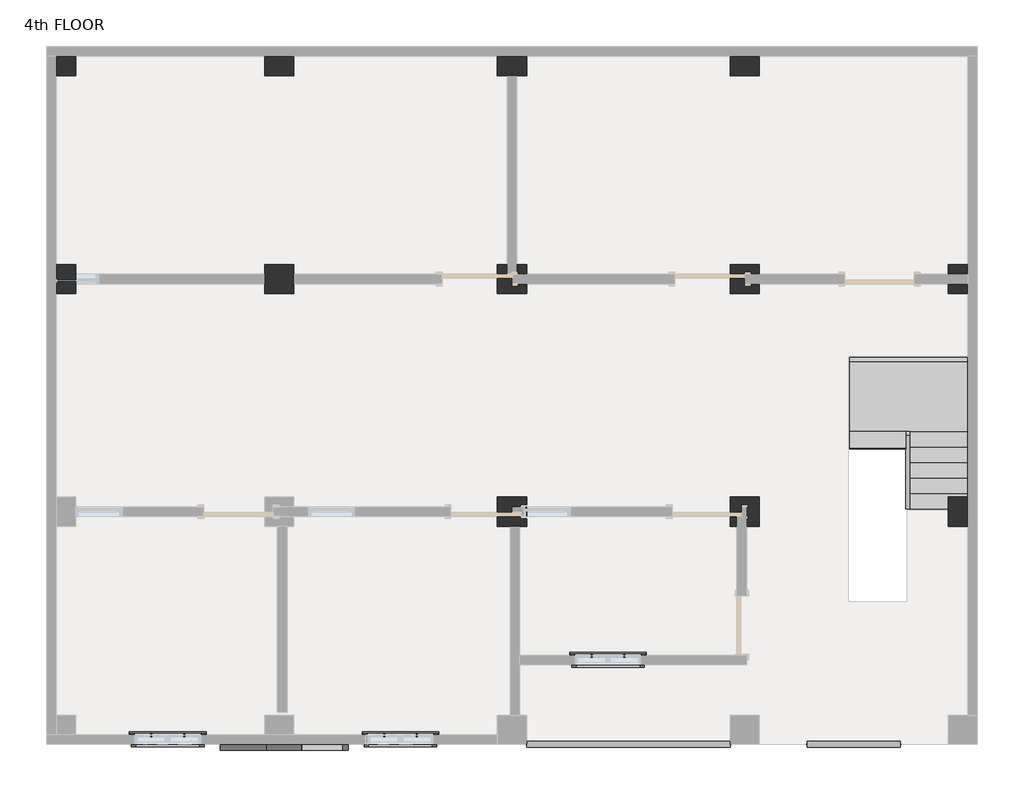
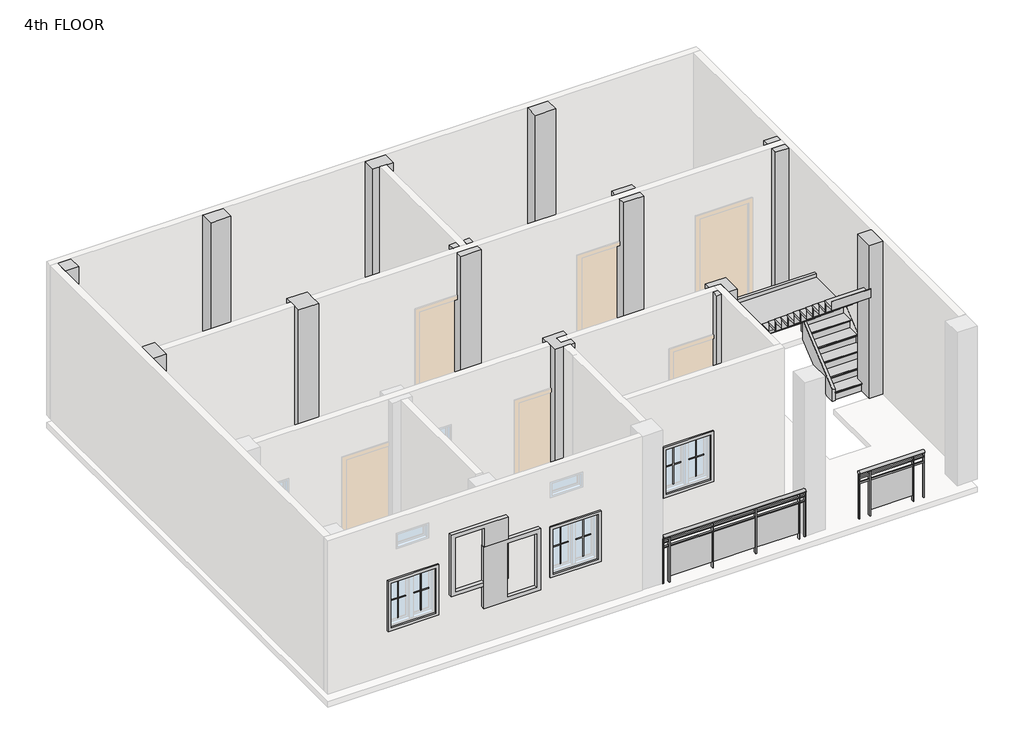
# One storey, part 2 of 2: 12 columns, 12 proxies, 4 members, 2 railings, 1 damper, 1 stair flight.
"""IFC4 building model written with IfcOpenShell, lengths in millimetres."""

from ifc_helpers import new_model, si_unit, point, frame, origin, place, context, project, spatial, polyline, ellipse_curve, trimmed, outline, extrude, faceted_brep, transform, mapped, element, save
from ifc_brep_helpers import plane_surface, extruded_surface, advanced_brep
from components import muntin_pattern_2x2_muntin_pattern_2x2_b3fe6957, muntin_pattern_2x2_muntin_pattern_2x2_3e0ecaf2, trim_window_exterior_flat_with_sill_41619996, trim_window_interior_flat_picture_frame_51c85655, duct_accessories_9_duct_accessories_1_ba76d1db, stair_flight_b92ce0aa

model = new_model("IFC4")

# Units and contexts
model_context = context("Model", 3, world=origin())
ifc_project = project(units=[si_unit("LENGTHUNIT", "METRE", prefix="MILLI")], contexts=[model_context])

# Site, building, storey
site = spatial("IfcSite", under=ifc_project)
building = spatial("IfcBuilding", under=site)
storey = spatial("IfcBuildingStorey", under=building, Name="4th FLOOR", Elevation=12039.6)

# Proxies
placement = place(None, origin())
muntin_pattern_2x2_muntin_pattern_2x2_shape = muntin_pattern_2x2_muntin_pattern_2x2_b3fe6957(model_context)
element("IfcBuildingElementProxy", 1, Name="Muntin Pattern_2x2 : Muntin Pattern_2x2", ObjectType="Muntin Pattern_2x2 : Muntin Pattern_2x2", at=placement, inside=storey, context=model_context, shape_type="MappedRepresentation", body=[
    mapped(muntin_pattern_2x2_muntin_pattern_2x2_shape, transform((-14441.409625, -253.8184478, 13023.85), x_axis=(1.0, 0.0, 0.0), y_axis=(0.0, 1.0, 0.0), z_axis=(0.0, 0.0, 1.0))),
])
element("IfcBuildingElementProxy", 2, Name="Muntin Pattern_2x2 : Muntin Pattern_2x2", ObjectType="Muntin Pattern_2x2 : Muntin Pattern_2x2", at=placement, inside=storey, context=model_context, shape_type="MappedRepresentation", body=[
    mapped(muntin_pattern_2x2_muntin_pattern_2x2_shape, transform((-11393.409625, -253.8184478, 13023.85), x_axis=(1.0, 0.0, 0.0), y_axis=(0.0, 1.0, 0.0), z_axis=(0.0, 0.0, 1.0))),
])
element("IfcBuildingElementProxy", 3, Name="Muntin Pattern_2x2 : Muntin Pattern_2x2", ObjectType="Muntin Pattern_2x2 : Muntin Pattern_2x2", at=placement, inside=storey, context=model_context, shape_type="MappedRepresentation", body=[
    mapped(muntin_pattern_2x2_muntin_pattern_2x2_shape, transform((-8675.609625, 787.5815522, 13023.85), x_axis=(1.0, 0.0, 0.0), y_axis=(0.0, 1.0, 0.0), z_axis=(0.0, 0.0, 1.0))),
])
muntin_pattern_2x2_muntin_pattern_2x2_2_shape = muntin_pattern_2x2_muntin_pattern_2x2_3e0ecaf2(model_context)
element("IfcBuildingElementProxy", 4, Name="Muntin Pattern_2x2 : Muntin Pattern_2x2", ObjectType="Muntin Pattern_2x2 : Muntin Pattern_2x2", at=placement, inside=storey, context=model_context, shape_type="MappedRepresentation", body=[
    mapped(muntin_pattern_2x2_muntin_pattern_2x2_2_shape, transform((-14012.784625, -253.8184478, 13023.85), x_axis=(-1.0, 0.0, 0.0), y_axis=(0.0, -1.0, 0.0), z_axis=(0.0, 0.0, 1.0))),
])
element("IfcBuildingElementProxy", 5, Name="Muntin Pattern_2x2 : Muntin Pattern_2x2", ObjectType="Muntin Pattern_2x2 : Muntin Pattern_2x2", at=placement, inside=storey, context=model_context, shape_type="MappedRepresentation", body=[
    mapped(muntin_pattern_2x2_muntin_pattern_2x2_2_shape, transform((-10964.784625, -253.8184478, 13023.85), x_axis=(-1.0, 0.0, 0.0), y_axis=(0.0, -1.0, 0.0), z_axis=(0.0, 0.0, 1.0))),
])
element("IfcBuildingElementProxy", 6, Name="Muntin Pattern_2x2 : Muntin Pattern_2x2", ObjectType="Muntin Pattern_2x2 : Muntin Pattern_2x2", at=placement, inside=storey, context=model_context, shape_type="MappedRepresentation", body=[
    mapped(muntin_pattern_2x2_muntin_pattern_2x2_2_shape, transform((-8246.984625, 787.5815522, 13023.85), x_axis=(-1.0, 0.0, 0.0), y_axis=(0.0, -1.0, 0.0), z_axis=(0.0, 0.0, 1.0))),
])
trim_window_exterior_flat_with_sill_shape = trim_window_exterior_flat_with_sill_41619996(model_context)
element("IfcBuildingElementProxy", 7, Name="Trim-Window-Exterior-Flat : with Sill", ObjectType="Trim-Window-Exterior-Flat : with Sill", at=placement, inside=storey, context=model_context, shape_type="MappedRepresentation", body=[
    mapped(trim_window_exterior_flat_with_sill_shape, transform((-14227.097125, -244.2934478, 13868.4), x_axis=(-1.0, 0.0, 0.0), y_axis=(0.0, 0.0, 1.0), z_axis=(0.0, 1.0, 0.0))),
])
element("IfcBuildingElementProxy", 8, Name="Trim-Window-Exterior-Flat : with Sill", ObjectType="Trim-Window-Exterior-Flat : with Sill", at=placement, inside=storey, context=model_context, shape_type="MappedRepresentation", body=[
    mapped(trim_window_exterior_flat_with_sill_shape, transform((-11179.097125, -244.2934478, 13868.4), x_axis=(-1.0, 0.0, 0.0), y_axis=(0.0, 0.0, 1.0), z_axis=(0.0, 1.0, 0.0))),
])
element("IfcBuildingElementProxy", 9, Name="Trim-Window-Exterior-Flat : with Sill", ObjectType="Trim-Window-Exterior-Flat : with Sill", at=placement, inside=storey, context=model_context, shape_type="MappedRepresentation", body=[
    mapped(trim_window_exterior_flat_with_sill_shape, transform((-8461.297125, 797.1065522, 13868.4), x_axis=(-1.0, 0.0, 0.0), y_axis=(0.0, 0.0, 1.0), z_axis=(0.0, 1.0, 0.0))),
])
trim_window_interior_flat_picture_frame_shape = trim_window_interior_flat_picture_frame_51c85655(model_context)
element("IfcBuildingElementProxy", 10, Name="Trim-Window-Interior-Flat : Picture Frame", ObjectType="Trim-Window-Interior-Flat : Picture Frame", at=placement, inside=storey, context=model_context, shape_type="MappedRepresentation", body=[
    mapped(trim_window_interior_flat_picture_frame_shape, transform((-14227.097125, -371.2934478, 13868.4), x_axis=(1.0, 0.0, 0.0), y_axis=(0.0, 0.0, 1.0), z_axis=(0.0, -1.0, 0.0))),
])
element("IfcBuildingElementProxy", 11, Name="Trim-Window-Interior-Flat : Picture Frame", ObjectType="Trim-Window-Interior-Flat : Picture Frame", at=placement, inside=storey, context=model_context, shape_type="MappedRepresentation", body=[
    mapped(trim_window_interior_flat_picture_frame_shape, transform((-11179.097125, -371.2934478, 13868.4), x_axis=(1.0, 0.0, 0.0), y_axis=(0.0, 0.0, 1.0), z_axis=(0.0, -1.0, 0.0))),
])
element("IfcBuildingElementProxy", 12, Name="Trim-Window-Interior-Flat : Picture Frame", ObjectType="Trim-Window-Interior-Flat : Picture Frame", at=placement, inside=storey, context=model_context, shape_type="MappedRepresentation", body=[
    mapped(trim_window_interior_flat_picture_frame_shape, transform((-8461.297125, 670.1065522, 13868.4), x_axis=(1.0, 0.0, 0.0), y_axis=(0.0, 0.0, 1.0), z_axis=(0.0, -1.0, 0.0))),
])

# Columns
element("IfcColumn", 13, ObjectType="column family : column family", at=placement, inside=storey, context=model_context, shape_type="SweptSolid", body=[
    extrude(outline(polyline([(-15433.597125, 8645.7065522), (-15433.597125, 8391.7065522), (-15687.597125, 8391.7065522), (-15687.597125, 8645.7065522), (-15433.597125, 8645.7065522)])), frame((0.0, 0.0, 12044.6), z_axis=(0.0, 0.0, 1.0), x_axis=(1.0, 0.0, 0.0)), (0.0, 0.0, 1.0), 3038.0),
])
element("IfcColumn", 14, ObjectType="column family : column family", at=placement, inside=storey, context=model_context, shape_type="SweptSolid", body=[
    extrude(outline(polyline([(-12576.097125, 5915.2065522), (-12576.097125, 5534.2065522), (-12957.097125, 5534.2065522), (-12957.097125, 5915.2065522), (-12576.097125, 5915.2065522)])), frame((0.0, 0.0, 12044.6), z_axis=(0.0, 0.0, 1.0), x_axis=(1.0, 0.0, 0.0)), (0.0, 0.0, 1.0), 3038.0),
])
element("IfcColumn", 15, ObjectType="column family : column family", at=placement, inside=storey, context=model_context, shape_type="Brep", body=[
    faceted_brep([(-9655.097125, 5915.2065522, 12044.6), (-9528.097125, 5915.2065522, 12044.6), (-9528.097125, 5788.2065522, 12044.6), (-9655.097125, 5788.2065522, 12044.6), (-9528.097125, 5915.2065522, 15082.6), (-9655.097125, 5915.2065522, 15082.6), (-9655.097125, 5788.2065522, 15082.6), (-9528.097125, 5788.2065522, 15082.6)], [[[0, 1, 2, 3]], [[4, 5, 6, 7]], [[0, 3, 6, 5]], [[4, 1, 0, 5]], [[3, 2, 7, 6]], [[1, 4, 7, 2]]]),
    faceted_brep([(-9528.097125, 5534.2065522, 15082.6), (-9528.097125, 5534.2065522, 12044.6), (-9528.097125, 5661.2065522, 12044.6), (-9528.097125, 5661.2065522, 15082.6), (-9909.097125, 5534.2065522, 12044.6), (-9909.097125, 5534.2065522, 15082.6), (-9909.097125, 5915.2065522, 12044.6), (-9909.097125, 5661.2065522, 15082.6), (-9909.097125, 5661.2065522, 14173.2), (-9909.097125, 5788.2065522, 14173.2), (-9909.097125, 5788.2065522, 15082.6), (-9909.097125, 5915.2065522, 15082.6), (-9782.097125, 5915.2065522, 15082.6), (-9782.097125, 5915.2065522, 12044.6), (-9782.097125, 5788.2065522, 12044.6), (-9782.097125, 5788.2065522, 15082.6), (-9782.097125, 5788.2065522, 14173.2), (-9718.597125, 5788.2065522, 12044.6), (-9718.597125, 5788.2065522, 14173.2), (-9718.597125, 5661.2065522, 12044.6), (-9718.597125, 5661.2065522, 14173.2)], [[[0, 1, 2, 3]], [[4, 1, 0, 5]], [[6, 4, 5, 7, 8, 9, 10, 11]], [[6, 11, 12, 13]], [[14, 13, 12, 15, 16]], [[17, 14, 16, 18]], [[19, 20, 8, 7, 3, 2]], [[1, 4, 6, 13, 14, 17, 19, 2]], [[5, 0, 3, 7]], [[12, 11, 10, 15]], [[9, 16, 15, 10]], [[18, 20, 19, 17]], [[20, 18, 16, 9, 8]]]),
])
element("IfcColumn", 16, ObjectType="column family : column family", at=placement, inside=storey, context=model_context, shape_type="Brep", body=[
    faceted_brep([(-6480.097125, 5534.2065522, 12044.6), (-6861.097125, 5534.2065522, 12044.6), (-6861.097125, 5915.2065522, 12044.6), (-6480.097125, 5915.2065522, 12044.6), (-6480.097125, 5788.2065522, 12044.6), (-6670.597125, 5788.2065522, 12044.6), (-6670.597125, 5661.2065522, 12044.6), (-6480.097125, 5661.2065522, 12044.6), (-6480.097125, 5534.2065522, 15082.6), (-6480.097125, 5661.2065522, 15082.6), (-6861.097125, 5534.2065522, 15082.6), (-6861.097125, 5661.2065522, 15082.6), (-6861.097125, 5661.2065522, 14173.2), (-6861.097125, 5788.2065522, 14173.2), (-6861.097125, 5788.2065522, 15082.6), (-6861.097125, 5915.2065522, 15082.6), (-6480.097125, 5915.2065522, 15082.6), (-6670.597125, 5661.2065522, 14173.2), (-6670.597125, 5788.2065522, 14173.2), (-6480.097125, 5788.2065522, 15082.6)], [[[0, 1, 2, 3, 4, 5, 6, 7]], [[8, 0, 7, 9]], [[1, 0, 8, 10]], [[2, 1, 10, 11, 12, 13, 14, 15]], [[3, 2, 15, 16]], [[10, 8, 9, 11]], [[6, 17, 12, 11, 9, 7]], [[13, 18, 5, 4, 19, 14]], [[3, 16, 19, 4]], [[16, 15, 14, 19]], [[18, 17, 6, 5]], [[17, 18, 13, 12]]]),
])
element("IfcColumn", 17, ObjectType="column family : column family", at=placement, inside=storey, context=model_context, shape_type="Brep", body=[
    faceted_brep([(-6480.097125, 2867.2065522, 12044.6), (-6480.097125, 2486.2065522, 12044.6), (-6645.197125, 2486.2065522, 12044.6), (-6645.197125, 2740.2065522, 12044.6), (-6708.697125, 2740.2065522, 12044.6), (-6708.697125, 2613.2065522, 12044.6), (-6772.197125, 2613.2065522, 12044.6), (-6772.197125, 2486.2065522, 12044.6), (-6861.097125, 2486.2065522, 12044.6), (-6861.097125, 2867.2065522, 12044.6), (-6480.097125, 2867.2065522, 15082.6), (-6480.097125, 2486.2065522, 15082.6), (-6861.097125, 2486.2065522, 15082.6), (-6772.197125, 2486.2065522, 15082.6), (-6861.097125, 2613.2065522, 15082.6), (-6861.097125, 2613.2065522, 14173.2), (-6861.097125, 2740.2065522, 14173.2), (-6861.097125, 2740.2065522, 15082.6), (-6861.097125, 2867.2065522, 15082.6), (-6772.197125, 2740.2065522, 15082.6), (-6645.197125, 2740.2065522, 15082.6), (-6645.197125, 2486.2065522, 15082.6), (-6772.197125, 2613.2065522, 15082.6), (-6772.197125, 2613.2065522, 14173.2), (-6772.197125, 2740.2065522, 14173.2), (-6708.697125, 2613.2065522, 14173.2), (-6708.697125, 2740.2065522, 14173.2)], [[[0, 1, 2, 3, 4, 5, 6, 7, 8, 9]], [[1, 0, 10, 11]], [[12, 8, 7, 13]], [[9, 8, 12, 14, 15, 16, 17, 18]], [[0, 9, 18, 10]], [[11, 10, 18, 17, 19, 20, 21]], [[15, 14, 22, 23]], [[17, 16, 24, 19]], [[20, 3, 2, 21]], [[6, 23, 22, 13, 7]], [[14, 12, 13, 22]], [[1, 11, 21, 2]], [[15, 23, 24, 16]], [[25, 23, 6, 5]], [[23, 25, 26, 24]], [[26, 25, 5, 4]], [[24, 26, 4, 3, 20, 19]]]),
])
element("IfcColumn", 18, ObjectType="column family : column family", at=placement, inside=storey, context=model_context, shape_type="Brep", body=[
    faceted_brep([(-9528.097125, 2486.2065522, 12044.6), (-9909.097125, 2486.2065522, 12044.6), (-9909.097125, 2867.2065522, 12044.6), (-9528.097125, 2867.2065522, 12044.6), (-9528.097125, 2740.2065522, 12044.6), (-9566.197125, 2740.2065522, 12044.6), (-9718.597125, 2740.2065522, 12044.6), (-9718.597125, 2613.2065522, 12044.6), (-9566.197125, 2613.2065522, 12044.6), (-9528.097125, 2613.2065522, 12044.6), (-9528.097125, 2486.2065522, 15082.6), (-9528.097125, 2613.2065522, 12344.4), (-9528.097125, 2740.2065522, 12344.4), (-9528.097125, 2867.2065522, 15082.6), (-9528.097125, 2740.2065522, 15082.6), (-9528.097125, 2740.2065522, 14173.2), (-9528.097125, 2613.2065522, 14173.2), (-9528.097125, 2613.2065522, 15082.6), (-9909.097125, 2486.2065522, 15082.6), (-9909.097125, 2867.2065522, 15082.6), (-9566.197125, 2613.2065522, 15082.6), (-9718.597125, 2613.2065522, 15082.6), (-9718.597125, 2740.2065522, 15082.6), (-9566.197125, 2740.2065522, 15082.6), (-9566.197125, 2613.2065522, 14173.2), (-9566.197125, 2613.2065522, 12344.4), (-9566.197125, 2740.2065522, 12344.4), (-9566.197125, 2740.2065522, 14173.2)], [[[0, 1, 2, 3, 4, 5, 6, 7, 8, 9]], [[10, 0, 9, 11, 12, 4, 3, 13, 14, 15, 16, 17]], [[1, 0, 10, 18]], [[2, 1, 18, 19]], [[3, 2, 19, 13]], [[18, 10, 17, 20, 21, 22, 23, 14, 13, 19]], [[11, 9, 8, 7, 21, 20, 17, 16, 24, 25]], [[4, 12, 26, 27, 15, 14, 23, 22, 6, 5]], [[21, 7, 6, 22]], [[25, 24, 27, 26]], [[25, 26, 12, 11]], [[27, 24, 16, 15]]]),
])
element("IfcColumn", 19, ObjectType="column family : column family", at=placement, inside=storey, context=model_context, shape_type="SweptSolid", body=[
    extrude(outline(polyline([(-12576.097125, 8391.7065522), (-12957.097125, 8391.7065522), (-12957.097125, 8645.7065522), (-12576.097125, 8645.7065522), (-12576.097125, 8391.7065522)])), frame((0.0, 0.0, 12044.6), z_axis=(0.0, 0.0, 1.0), x_axis=(1.0, 0.0, 0.0)), (0.0, 0.0, 1.0), 3038.0),
])
element("IfcColumn", 20, ObjectType="column family : column family", at=placement, inside=storey, context=model_context, shape_type="SweptSolid", body=[
    extrude(outline(polyline([(-9528.097125, 8391.7065522), (-9909.097125, 8391.7065522), (-9909.097125, 8645.7065522), (-9528.097125, 8645.7065522), (-9528.097125, 8391.7065522)])), frame((0.0, 0.0, 12044.6), z_axis=(0.0, 0.0, 1.0), x_axis=(1.0, 0.0, 0.0)), (0.0, 0.0, 1.0), 3038.0),
])
element("IfcColumn", 21, ObjectType="column family : column family", at=placement, inside=storey, context=model_context, shape_type="SweptSolid", body=[
    extrude(outline(polyline([(-6480.097125, 8391.7065522), (-6861.097125, 8391.7065522), (-6861.097125, 8645.7065522), (-6480.097125, 8645.7065522), (-6480.097125, 8391.7065522)])), frame((0.0, 0.0, 12044.6), z_axis=(0.0, 0.0, 1.0), x_axis=(1.0, 0.0, 0.0)), (0.0, 0.0, 1.0), 3038.0),
])
element("IfcColumn", 22, ObjectType="column family : column family", at=placement, inside=storey, context=model_context, shape_type="SweptSolid", body=[
    extrude(outline(polyline([(-4003.597125, 5915.2065522), (-3749.597125, 5915.2065522), (-3749.597125, 5788.2065522), (-4003.597125, 5788.2065522), (-4003.597125, 5915.2065522)])), frame((0.0, 0.0, 12044.6), z_axis=(0.0, 0.0, 1.0), x_axis=(1.0, 0.0, 0.0)), (0.0, 0.0, 1.0), 3038.0),
    extrude(outline(polyline([(-3749.597125, 5534.2065522), (-4003.597125, 5534.2065522), (-4003.597125, 5661.2065522), (-3749.597125, 5661.2065522), (-3749.597125, 5534.2065522)])), frame((0.0, 0.0, 12044.6), z_axis=(0.0, 0.0, 1.0), x_axis=(1.0, 0.0, 0.0)), (0.0, 0.0, 1.0), 3038.0),
])
element("IfcColumn", 23, ObjectType="column family : column family", at=placement, inside=storey, context=model_context, shape_type="SweptSolid", body=[
    extrude(outline(polyline([(-4003.597125, 2486.2065522), (-4003.597125, 2867.2065522), (-3749.597125, 2867.2065522), (-3749.597125, 2486.2065522), (-4003.597125, 2486.2065522)])), frame((0.0, 0.0, 12044.6), z_axis=(0.0, 0.0, 1.0), x_axis=(1.0, 0.0, 0.0)), (0.0, 0.0, 1.0), 3038.0),
])
element("IfcColumn", 24, ObjectType="column family : column family", at=placement, inside=storey, context=model_context, shape_type="SweptSolid", body=[
    extrude(outline(polyline([(-15433.597125, 5915.2065522), (-15433.597125, 5534.2065522), (-15687.597125, 5534.2065522), (-15687.597125, 5915.2065522), (-15433.597125, 5915.2065522)])), frame((0.0, 0.0, 12044.6), z_axis=(0.0, 0.0, 1.0), x_axis=(1.0, 0.0, 0.0)), (0.0, 0.0, 1.0), 3038.0),
])

# Damper
duct_accessories_9_duct_accessories_1_shape = duct_accessories_9_duct_accessories_1_ba76d1db(model_context)
element("IfcDamper", 25, ObjectType="Duct Accessories 9 : Duct Accessories 1", at=placement, inside=storey, context=model_context, shape_type="MappedRepresentation", body=[
    mapped(duct_accessories_9_duct_accessories_1_shape, transform((0.0, 0.0, 0.0), x_axis=(1.0, 0.0, 0.0), y_axis=(0.0, 1.0, 0.0), z_axis=(0.0, 0.0, 1.0))),
])

# Members
element("IfcMember", 26, ObjectType="Stringer - 2\" Width", at=placement, inside=storey, context=model_context, shape_type="SweptSolid", body=[
    extrude(outline(polyline([(2714.6319226, 12039.6), (2714.6319226, 12276.4438745), (3679.8319226, 13080.7772078), (3679.8319226, 12684.0165243), (2906.5320935, 12039.6), (2714.6319226, 12039.6)])), frame((-4563.0136682, 0.0, 0.0), z_axis=(1.0, 0.0, 0.0), x_axis=(0.0, 1.0, 0.0)), (0.0, 0.0, 1.0), 50.8),
])
element("IfcMember", 27, ObjectType="Stringer - 2\" Width", at=placement, inside=storey, context=model_context, shape_type="SweptSolid", body=[
    extrude(outline(polyline([(-4512.2136682, 3730.6319226), (-4512.2136682, 3679.8319226), (-4563.0136682, 3679.8319226), (-4563.0136682, 3730.6319226), (-4512.2136682, 3730.6319226)])), frame((0.0, 0.0, 12827.0), z_axis=(0.0, 0.0, 1.0), x_axis=(1.0, 0.0, 0.0)), (0.0, 0.0, 1.0), 304.8),
])
element("IfcMember", 28, ObjectType="Stringer - 2\" Width", at=placement, inside=storey, context=model_context, shape_type="SweptSolid", body=[
    extrude(outline(polyline([(2714.6319226, 12039.6), (2714.6319226, 12276.4438745), (3741.0592732, 13131.8), (4217.1720935, 13131.8), (2906.5320935, 12039.6), (2714.6319226, 12039.6)])), frame((-3749.597125, 0.0, 0.0), z_axis=(1.0, 0.0, 0.0), x_axis=(0.0, 1.0, 0.0)), (0.0, 0.0, 1.0), 50.8),
])
element("IfcMember", 29, ObjectType="Stringer - 2\" Width", at=placement, inside=storey, context=model_context, shape_type="SweptSolid", body=[
    extrude(outline(polyline([(-3698.797125, 4695.8319226), (-3698.797125, 4645.0319226), (-5295.0246464, 4645.0319226), (-5295.0246464, 4695.8319226), (-3698.797125, 4695.8319226)])), frame((0.0, 0.0, 12827.0), z_axis=(0.0, 0.0, 1.0), x_axis=(1.0, 0.0, 0.0)), (0.0, 0.0, 1.0), 304.8),
])

# Railings
element("IfcRailing", 30, ObjectType="Glass Panel - Bottom Fill", at=placement, inside=storey, context=model_context, shape_type="SolidModel", body=[
    advanced_brep(
    [(-9528.097125, -333.1934478, 12954.0), (-9528.097125, -409.3934478, 12954.0), (-6861.097125, -333.1934478, 12954.0), (-6861.097125, -409.3934478, 12954.0)],
    [
        (0, 1, ellipse_curve(frame((-9528.097125, -371.2934478, 12954.0), z_axis=(-1.0, 0.0, 0.0), x_axis=(0.0, -1.0, 0.0)), 38.1, 28.575)),
        (1, 0, ellipse_curve(frame((-9528.097125, -371.2934478, 12954.0), z_axis=(-1.0, 0.0, 0.0), x_axis=(0.0, -1.0, 0.0)), 38.1, 28.575)),
        (2, 3, ellipse_curve(frame((-6861.097125, -371.2934478, 12954.0), z_axis=(1.0, 0.0, 0.0), x_axis=(0.0, -1.0, 0.0)), 38.1, 28.575)),
        (3, 2, ellipse_curve(frame((-6861.097125, -371.2934478, 12954.0), z_axis=(1.0, 0.0, 0.0), x_axis=(0.0, -1.0, 0.0)), 38.1, 28.575)),
        (0, 2),
        (3, 1),
    ],
    [
        plane_surface(frame((-9528.097125, -371.2934478, 12954.0), z_axis=(-1.0, 0.0, 0.0), x_axis=(0.0, 1.0, 0.0))),
        plane_surface(frame((-6861.097125, -371.2934478, 12954.0), z_axis=(1.0, 0.0, 0.0), x_axis=(0.0, 1.0, 0.0))),
        extruded_surface(trimmed(ellipse_curve(frame((-6861.097125, -371.2934478, 12954.0), z_axis=(-1.0, 0.0, 0.0), x_axis=(0.0, -1.0, 0.0)), 38.1, 28.575), [point((-6861.097125, -333.1934478, 12954.0))], [point((-6861.097125, -409.3934478, 12954.0))], True, "CARTESIAN"), (-2667.0, 0.0, 0.0), 2667.0),
        extruded_surface(trimmed(ellipse_curve(frame((-6861.097125, -371.2934478, 12954.0), z_axis=(-1.0, 0.0, 0.0), x_axis=(0.0, -1.0, 0.0)), 38.1, 28.575), [point((-6861.097125, -409.3934478, 12954.0))], [point((-6861.097125, -333.1934478, 12954.0))], True, "CARTESIAN"), (-2667.0, 0.0, 0.0), 2667.0),
    ],
    [
        (0, [[1, 2]]),
        (1, [[3, 4]]),
        (2, [[-1, 5, -4, 6]]),
        (3, [[-2, -6, -3, -5]]),
    ],
),
    extrude(outline(polyline([(-9528.097125, -383.9934478), (-9528.097125, -358.5934478), (-6861.097125, -358.5934478), (-6861.097125, -383.9934478), (-9528.097125, -383.9934478)])), frame((0.0, 0.0, 12839.7), z_axis=(0.0, 0.0, 1.0), x_axis=(1.0, 0.0, 0.0)), (0.0, 0.0, 1.0), 25.4),
    extrude(outline(polyline([(-9528.097125, -383.9934478), (-9528.097125, -358.5934478), (-6861.097125, -358.5934478), (-6861.097125, -383.9934478), (-9528.097125, -383.9934478)])), frame((0.0, 0.0, 12738.1), z_axis=(0.0, 0.0, 1.0), x_axis=(1.0, 0.0, 0.0)), (0.0, 0.0, 1.0), 25.4),
    extrude(outline(polyline([(-6981.747125, -396.6934478), (-6981.747125, -345.8934478), (-6969.047125, -345.8934478), (-6969.047125, -396.6934478), (-6981.747125, -396.6934478)])), frame((0.0, 0.0, 12039.6), z_axis=(0.0, 0.0, 1.0), x_axis=(1.0, 0.0, 0.0)), (0.0, 0.0, 1.0), 885.6788223),
    extrude(outline(polyline([(-7788.197125, -364.7582908), (-6975.397125, -364.7582908), (-6975.397125, -371.1082908), (-7788.197125, -371.1082908), (-7788.197125, -364.7582908)])), frame((0.0, 0.0, 12141.2), z_axis=(0.0, 0.0, 1.0), x_axis=(1.0, 0.0, 0.0)), (0.0, 0.0, 1.0), 596.9),
    extrude(outline(polyline([(-7794.547125, -396.6934478), (-7794.547125, -345.8934478), (-7781.847125, -345.8934478), (-7781.847125, -396.6934478), (-7794.547125, -396.6934478)])), frame((0.0, 0.0, 12039.6), z_axis=(0.0, 0.0, 1.0), x_axis=(1.0, 0.0, 0.0)), (0.0, 0.0, 1.0), 885.6788223),
    extrude(outline(polyline([(-8600.997125, -364.7582908), (-7788.197125, -364.7582908), (-7788.197125, -371.1082908), (-8600.997125, -371.1082908), (-8600.997125, -364.7582908)])), frame((0.0, 0.0, 12141.2), z_axis=(0.0, 0.0, 1.0), x_axis=(1.0, 0.0, 0.0)), (0.0, 0.0, 1.0), 596.9),
    extrude(outline(polyline([(-8607.347125, -396.6934478), (-8607.347125, -345.8934478), (-8594.647125, -345.8934478), (-8594.647125, -396.6934478), (-8607.347125, -396.6934478)])), frame((0.0, 0.0, 12039.6), z_axis=(0.0, 0.0, 1.0), x_axis=(1.0, 0.0, 0.0)), (0.0, 0.0, 1.0), 885.6788223),
    extrude(outline(polyline([(-9413.797125, -364.7582908), (-8600.997125, -364.7582908), (-8600.997125, -371.1082908), (-9413.797125, -371.1082908), (-9413.797125, -364.7582908)])), frame((0.0, 0.0, 12141.2), z_axis=(0.0, 0.0, 1.0), x_axis=(1.0, 0.0, 0.0)), (0.0, 0.0, 1.0), 596.9),
    extrude(outline(polyline([(-9420.147125, -396.6934478), (-9420.147125, -345.8934478), (-9407.447125, -345.8934478), (-9407.447125, -396.6934478), (-9420.147125, -396.6934478)])), frame((0.0, 0.0, 12039.6), z_axis=(0.0, 0.0, 1.0), x_axis=(1.0, 0.0, 0.0)), (0.0, 0.0, 1.0), 885.6788223),
    extrude(outline(polyline([(-6873.797125, -380.8184478), (-6873.797125, -361.7684478), (-6854.747125, -361.7684478), (-6854.747125, -380.8184478), (-6873.797125, -380.8184478)])), frame((0.0, 0.0, 12039.6), z_axis=(0.0, 0.0, 1.0), x_axis=(1.0, 0.0, 0.0)), (0.0, 0.0, 1.0), 885.6788223),
    extrude(outline(polyline([(-9534.447125, -380.8184478), (-9534.447125, -361.7684478), (-9515.397125, -361.7684478), (-9515.397125, -380.8184478), (-9534.447125, -380.8184478)])), frame((0.0, 0.0, 12039.6), z_axis=(0.0, 0.0, 1.0), x_axis=(1.0, 0.0, 0.0)), (0.0, 0.0, 1.0), 885.6788223),
])
element("IfcRailing", 31, ObjectType="Glass Panel - Bottom Fill", at=placement, inside=storey, context=model_context, shape_type="SolidModel", body=[
    advanced_brep(
    [(-5851.447125, -333.1934478, 12954.0), (-5851.447125, -409.3934478, 12954.0), (-4632.247125, -333.1934478, 12954.0), (-4632.247125, -409.3934478, 12954.0)],
    [
        (0, 1, ellipse_curve(frame((-5851.447125, -371.2934478, 12954.0), z_axis=(-1.0, 0.0, 0.0), x_axis=(0.0, -1.0, 0.0)), 38.1, 28.575)),
        (1, 0, ellipse_curve(frame((-5851.447125, -371.2934478, 12954.0), z_axis=(-1.0, 0.0, 0.0), x_axis=(0.0, -1.0, 0.0)), 38.1, 28.575)),
        (2, 3, ellipse_curve(frame((-4632.247125, -371.2934478, 12954.0), z_axis=(1.0, 0.0, 0.0), x_axis=(0.0, -1.0, 0.0)), 38.1, 28.575)),
        (3, 2, ellipse_curve(frame((-4632.247125, -371.2934478, 12954.0), z_axis=(1.0, 0.0, 0.0), x_axis=(0.0, -1.0, 0.0)), 38.1, 28.575)),
        (0, 2),
        (3, 1),
    ],
    [
        plane_surface(frame((-5851.447125, -371.2934478, 12954.0), z_axis=(-1.0, 0.0, 0.0), x_axis=(0.0, 1.0, 0.0))),
        plane_surface(frame((-4632.247125, -371.2934478, 12954.0), z_axis=(1.0, 0.0, 0.0), x_axis=(0.0, 1.0, 0.0))),
        extruded_surface(trimmed(ellipse_curve(frame((-4632.247125, -371.2934478, 12954.0), z_axis=(-1.0, 0.0, 0.0), x_axis=(0.0, -1.0, 0.0)), 38.1, 28.575), [point((-4632.247125, -333.1934478, 12954.0))], [point((-4632.247125, -409.3934478, 12954.0))], True, "CARTESIAN"), (-1219.1999999999998, 0.0, 0.0), 1219.1999999999998),
        extruded_surface(trimmed(ellipse_curve(frame((-4632.247125, -371.2934478, 12954.0), z_axis=(-1.0, 0.0, 0.0), x_axis=(0.0, -1.0, 0.0)), 38.1, 28.575), [point((-4632.247125, -409.3934478, 12954.0))], [point((-4632.247125, -333.1934478, 12954.0))], True, "CARTESIAN"), (-1219.1999999999998, 0.0, 0.0), 1219.1999999999998),
    ],
    [
        (0, [[1, 2]]),
        (1, [[3, 4]]),
        (2, [[-1, 5, -4, 6]]),
        (3, [[-2, -6, -3, -5]]),
    ],
),
    extrude(outline(polyline([(-5851.447125, -383.9934478), (-5851.447125, -358.5934478), (-4632.247125, -358.5934478), (-4632.247125, -383.9934478), (-5851.447125, -383.9934478)])), frame((0.0, 0.0, 12839.7), z_axis=(0.0, 0.0, 1.0), x_axis=(1.0, 0.0, 0.0)), (0.0, 0.0, 1.0), 25.4),
    extrude(outline(polyline([(-5851.447125, -383.9934478), (-5851.447125, -358.5934478), (-4632.247125, -358.5934478), (-4632.247125, -383.9934478), (-5851.447125, -383.9934478)])), frame((0.0, 0.0, 12738.1), z_axis=(0.0, 0.0, 1.0), x_axis=(1.0, 0.0, 0.0)), (0.0, 0.0, 1.0), 25.4),
    extrude(outline(polyline([(-4841.797125, -396.6934478), (-4841.797125, -345.8934478), (-4829.097125, -345.8934478), (-4829.097125, -396.6934478), (-4841.797125, -396.6934478)])), frame((0.0, 0.0, 12039.6), z_axis=(0.0, 0.0, 1.0), x_axis=(1.0, 0.0, 0.0)), (0.0, 0.0, 1.0), 885.6788223),
    extrude(outline(polyline([(-5648.247125, -364.7582908), (-4835.447125, -364.7582908), (-4835.447125, -371.1082908), (-5648.247125, -371.1082908), (-5648.247125, -364.7582908)])), frame((0.0, 0.0, 12141.2), z_axis=(0.0, 0.0, 1.0), x_axis=(1.0, 0.0, 0.0)), (0.0, 0.0, 1.0), 596.9),
    extrude(outline(polyline([(-5654.597125, -396.6934478), (-5654.597125, -345.8934478), (-5641.897125, -345.8934478), (-5641.897125, -396.6934478), (-5654.597125, -396.6934478)])), frame((0.0, 0.0, 12039.6), z_axis=(0.0, 0.0, 1.0), x_axis=(1.0, 0.0, 0.0)), (0.0, 0.0, 1.0), 885.6788223),
    extrude(outline(polyline([(-4644.947125, -380.8184478), (-4644.947125, -361.7684478), (-4625.897125, -361.7684478), (-4625.897125, -380.8184478), (-4644.947125, -380.8184478)])), frame((0.0, 0.0, 12039.6), z_axis=(0.0, 0.0, 1.0), x_axis=(1.0, 0.0, 0.0)), (0.0, 0.0, 1.0), 885.6788223),
    extrude(outline(polyline([(-5857.797125, -380.8184478), (-5857.797125, -361.7684478), (-5838.747125, -361.7684478), (-5838.747125, -380.8184478), (-5857.797125, -380.8184478)])), frame((0.0, 0.0, 12039.6), z_axis=(0.0, 0.0, 1.0), x_axis=(1.0, 0.0, 0.0)), (0.0, 0.0, 1.0), 885.6788223),
])

# Stair flight
stair_flight_shape = stair_flight_b92ce0aa(model_context)
element("IfcStairFlight", 32, ObjectType="2\" Tread 1\" Nosing 1/4\" Riser", at=placement, inside=storey, context=model_context, shape_type="MappedRepresentation", body=[
    mapped(stair_flight_shape, transform((0.0, 0.0, 0.0), x_axis=(1.0, 0.0, 0.0), y_axis=(0.0, 1.0, 0.0), z_axis=(0.0, 0.0, 1.0))),
])

save(model, "model.ifc")

# Revit data of these elements
# Type "Muntin Pattern_2x2 : Muntin Pattern_2x2"
#   Width [instance default] = 4' - 0"
#   Thickness = 0' - 0 1/2"
#   Height [instance default] = 4' - 0"
#   Distance = 0' - 0 3/4"
#   Interior Material [instance default] = none
#   Exterior Material [instance default] = none
#   Default Elevation = 0
# Type "Trim-Window-Exterior-Flat : with Sill"
#   Trim Width = 0' - 2 1/4"
#   Trim Thickness_Picture Frame = 0' - 1 1/4"
#   Trim Thickness_with Sill = 0' - 0 3/4"
#   Sill Thickness = 0' - 1 1/4"
#   Opening Width [instance default] = 2' - 0"
#   Opening Height [instance default] = 3' - 0"
#   Default Elevation = 4' - 0"
#   Sill = yes
#   Picture Frame = no
#   Trim Material [instance default] = none
# Type "Trim-Window-Interior-Flat : Picture Frame"
#   Trim Thickness_Picture Frame = 0' - 1 1/4"
#   Trim Width = 0' - 2 1/4"
#   Trim Thickness_with Sill = 0' - 0 3/4"
#   Sill Thickness = 0' - 1 1/4"
#   Opening Width [instance default] = 2' - 0"
#   Opening Height [instance default] = 3' - 0"
#   Default Elevation = 4' - 0"
#   Sill = no
#   Picture Frame = yes
#   Trim Material [instance default] = none
# Type "column family : column family"
#   w2 [instance default] = 0' - 9.88189"
#   w1 [instance default] = 0' - 9.01575"
#   Depth = 1' - 11.62205"
#   Width = 1' - 11.62205"
# Type "Glass Panel - Bottom Fill"
#   Assembly Code = "C2010400"
#   built-in parameter 1008612 = 0.0416667 (stored number, unit not read)
#   built-in parameter 1008611 = 0.0416667 (stored number, unit not read)
#   built-in parameter 1008609 = 0.333333 (stored number, unit not read)
#   built-in parameter 1008604 = 0.166667 (stored number, unit not read)
#   built-in parameter 1008603 = 0.166667 (stored number, unit not read)
#   Railing Height = 3' - 0"
#   built-in parameter 1008630 = 2
#   built-in parameter 1008610 = 2
#   built-in parameter 1008618 = Baluster - Square : 3/4"
# Elements 1, 2, 3, 4, 5, 6 (IfcBuildingElementProxy, "Muntin Pattern_2x2 : Muntin Pattern_2x2")
#   Width = 0' - 11 5/8"
#   Height = 2' - 6 1/2"
#   Interior Material = Wood - Stained
#   Exterior Material = Clad - White
#   Phase Created = New Construction
#   Materials on its faces: "Clad - White", "Wood - Stained"
# Elements 7, 8, 9 (IfcBuildingElementProxy, "Trim-Window-Exterior-Flat : with Sill")
#   Opening Width = 2' - 10"
#   Opening Height = 3' - 0"
#   Trim Material = Clad - White
#   Phase Created = New Construction
#   Materials on its faces: "Clad - White"
# Elements 10, 11, 12 (IfcBuildingElementProxy, "Trim-Window-Interior-Flat : Picture Frame")
#   Opening Width = 2' - 10"
#   Opening Height = 3' - 0"
#   Trim Material = Wood - Stained
#   Phase Created = New Construction
#   Materials on its faces: "Wood - Stained"
# Elements 13, 14, 15, 19, 20, 21 (IfcColumn, "column family : column family")
#   w2 = 1' - 3"
#   w1 = 1' - 3"
#   Phase Created = New Construction
#   Materials on its faces: "Default Wall"
# Elements 16, 22, 23 (IfcColumn, "column family : column family")
#   w2 = 1' - 3"
#   w1 = 1' - 3"
#   Phase Created = New Construction
#   Materials on its faces: "grey", "Default Wall"
# Elements 17, 18 (IfcColumn, "column family : column family")
#   w2 = 1' - 3"
#   w1 = 1' - 3"
#   Phase Created = New Construction
#   Materials on its faces: "Default Wall", "inside wall"
# Element 24 (IfcColumn, "column family : column family")
#   w2 = 1' - 3"
#   w1 = 1' - 3"
#   Phase Created = New Construction
#   Materials on its faces: "inside wall", "Default Wall"
# Element 25 (IfcDamper, "Duct Accessories 9 : Duct Accessories 1")
#   Mark = "9"
#   Phase Created = New Construction
#   Materials on its faces: "border"
# Elements 26, 27, 28, 29 (IfcMember, "Stringer - 2\" Width")
#   Phase Created = New Construction
# Elements 30, 31 (IfcRailing, "Glass Panel - Bottom Fill")
#   Phase Created = New Construction
#   Materials on its faces: "Glass"
# Element 32 (IfcStairFlight, "2\" Tread 1\" Nosing 1/4\" Riser")
#   Phase Created = New Construction
# Materials
#   "Clad - White": class "Wood", colour RGB 242 242 238, transparency 0, Cost = 0
#   "Wood - Stained": class "Wood", colour RGB 224 178 126, transparency 0, Cost = 0
#   "Default Wall": colour RGB 128 128 128, transparency 0, Cost = 0
#   "grey": class "Generic", colour RGB 80 80 80, transparency 0, Cost = 0
#   "inside wall": class "Generic", colour RGB 199 224 95, transparency 0, Cost = 0
#   "border": class "Generic", colour RGB 144 144 144, transparency 0, Cost = 0
#   "Glass": class "Glass", colour RGB 0 128 192, transparency 0.75, Description = "Soda Lime Glass", Cost = 0
